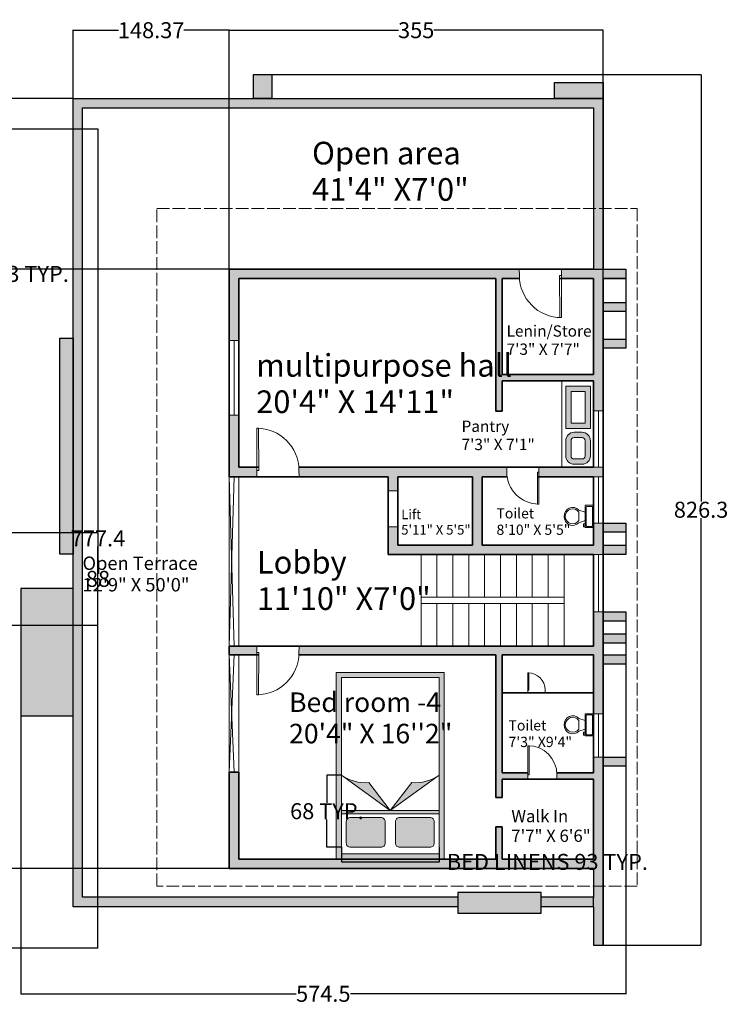
# Model space of a CAD drawing. Units: inches. Extents: x -828 to 1568, y -491 to 539.
# Tile 6 of 6: x 895 to 1568, y -470 to 464. Entities that reach past the tile are written whole.
import ezdxf

# ---------------------------------------------------------------- set-up
doc = ezdxf.new("R2010")
doc.units = ezdxf.units.IN
doc.header["$MEASUREMENT"] = 0
doc.linetypes.add('ACAD_ISO02W100', pattern=[15, 12, -3])
for name, color, linetype, lineweight in [('A-ANNO-DIMS', 2, 'Continuous', 18), ('A-AREA-IDEN', 7, 'Continuous', 18), ('A-DOOR', 3, 'Continuous', 18), ('A-FLOR-CASE', 9, 'Continuous', 18), ('A-FLOR-EVTR', 4, 'Continuous', 18), ('A-FLOR-FIXT', 9, 'Continuous', 18), ('A-FLOR-FIXT-PATT', 253, 'Continuous', 13), ('A-FLOR-SHFT', 7, 'Continuous', 25), ('A-FLOR-STRS', 7, 'Continuous', 18), ('A-FURN', 8, 'Continuous', 18), ('A-FURN-PATT', 253, 'Continuous', 13), ('A-GLAZ', 4, 'Continuous', 18), ('A-ROOF-OVHD', 8, 'ACAD_ISO02W100', 13), ('A-ROOF-PATT', 8, 'Continuous', 13), ('A-ROOF-PRPT', 7, 'Continuous', 25), ('A-WALL', 7, 'Continuous', 35), ('A-WALL-PATT', 8, 'Continuous', 13)]:
    doc.layers.add(name, color=color, linetype=linetype, lineweight=lineweight)
doc.styles.get("Standard").update_dxf_attribs({"font": 'arial.ttf'})
doc.dimstyles.get("Standard").update_dxf_attribs({"dimtxt": 15.18, "dimasz": 0.18, "dimexe": 0.18, "dimexo": 0.0625, "dimgap": 0.09, "dimtad": 0, "dimtih": 1, "dimtoh": 1, "dimdec": 0, "dimzin": 0, "dimdsep": 46, "dimlunit": 3, "dimtxsty": 'Standard', "dimcen": 0.09, "dimadec": 0, "dimazin": 0, "dimtfac": 1, "dimtdec": 0, "dimtofl": 0, "dimtmove": 0, "dimatfit": 3, "dimfxl": 1, "dimtolj": 1, "dimtzin": 0, "dimarcsym": 0})

# ---------------------------------------------------------------- blocks, each defined once
blk = doc.blocks.new('*U2')
for p, q in [((0, 0), (0, -6)), ((40, 0), (40, -6))]:
    blk.add_line(p, q)
blk.add_lwpolyline([(0, 0), (0, 40), (1.75, 40), (1.75, 0)], close=True)
blk.add_arc((0, 0), 40, 0, 90)
blk = doc.blocks.new('*U6')
for p, q in [((-10, -8.5), (-8, -8.5)), ((-10, -9.5), (-10, -8.5)), ((-8, -8.5), (-8, -8)), ((-7, -8), (-7, -9.5)), ((-4, -8), (-6, -14)), ((4, -8), (6, -14)), ((9.5, -6), (9.5, -2)), ((-7, -9.5), (-10, -9.5)), ((4, -14), (-4, -14))]:
    blk.add_line(p, q)
blk.add_lwpolyline([(10.5, -8), (10.5, 0), (-10.5, 0), (-10.5, -8)], close=True)
for points in [[(-9.5, -2), (-9.5, -6)], [(8.5, -1), (-8.5, -1)], [(-8.5, -7), (8.5, -7)]]:
    blk.add_lwpolyline(points)
for centre, radius, start, end in [((-8.625, -1.875), 0.8839, 81.8699, 188.1301), ((-8.625, -6.125), 0.8839, 171.869898, 278.1301), ((8.625, -1.875), 0.8839, 351.8699, 98.1301), ((8.625, -6.125), 0.8839, 261.8699, 8.1301), ((-0.4772, -19.9188), 8.0953, 133.01722, 273.38), ((0.0374, -19.8731), 7.127, 124.50543, 269.7), ((-0.0373, -19.8731), 7.127, 270.3, 55.4946), ((0.4773, -19.9188), 8.0953, 266.62, 46.9828)]:
    blk.add_arc(centre, radius, start, end)
blk = doc.blocks.new('BED-LINENS-DOUBLE')
h = blk.add_hatch(color=256)
h.dxf.hatch_style = 1
h.paths.add_polyline_path([(0, 92.62, -0.182673), (7.08, 66.8), (33.7, 46.31)])
h.paths.add_polyline_path([(33.7, 46.31), (7.08, 25.82, -0.182673), (0, 0)])
h = blk.add_hatch(color=256)
h.dxf.hatch_style = 1
h.paths.add_polyline_path([(36.7, 46.31), (33.7, 46.31), (33.7, 0), (36.7, 0)])
h.paths.add_polyline_path([(36.7, 92.62), (33.7, 92.62), (33.7, 46.31), (36.7, 46.31)])
h = blk.add_hatch(color=256)
h.dxf.hatch_style = 1
h.paths.add_polyline_path([(68.49, 84.07, 0.414214), (64.49, 88.07), (44.24, 88.07, 0.414214), (40.24, 84.07), (40.24, 55.21, 0.414214), (44.24, 51.21), (64.49, 51.21, 0.414214), (68.49, 55.21)])
h = blk.add_hatch(color=256)
h.dxf.hatch_style = 1
h.paths.add_polyline_path([(68.49, 37.42, 0.414214), (64.49, 41.42), (44.24, 41.42, 0.414214), (40.24, 37.42), (40.24, 8.55, 0.414214), (44.24, 4.55), (64.49, 4.55, 0.414214), (68.49, 8.55)])
for p, q in [((33.7, 46.31), (0, 92.62)), ((33.7, 0), (33.7, 92.62)), ((36.7, 0), (36.7, 92.62)), ((33.7, 46.31), (7.08, 66.8)), ((33.7, 46.31), (0, 0)), ((33.7, 46.31), (7.08, 25.82))]:
    blk.add_line(p, q)
for points in [[(64.49, 51.21), (44.24, 51.21, -0.414214), (40.24, 55.21), (40.24, 84.07, -0.414214), (44.24, 88.07), (64.49, 88.07, -0.414214), (68.49, 84.07), (68.49, 55.21, -0.414214)], [(64.49, 41.42), (44.24, 41.42, 0.414214), (40.24, 37.42), (40.24, 8.55, 0.414214), (44.24, 4.55), (64.49, 4.55, 0.414214), (68.49, 8.55), (68.49, 37.42, 0.414214)]]:
    blk.add_lwpolyline(points, format="xyb", close=True)
for centre, start, end in [((-30.62, 70.34), 354.63295, 36.04187), ((-30.62, 22.28), 323.95813, 5.36705)]:
    blk.add_arc(centre, 37.87, start, end)
blk = doc.blocks.new('*D25')
at = {"layer": 'A-ANNO-DIMS', "color": 0, "lineweight": -2, "transparency": 16777216}
for p, q in [((822.84, 244.58), (829.43, 244.58)), ((829.25, 244.4), (829.25, 230.97)), ((829.25, 201.64), (829.25, 215.08)), ((822.84, 201.46), (829.43, 201.46))]:
    blk.add_line(p, q, dxfattribs=at)
at = {"layer": 'A-ANNO-DIMS', "color": 0, "lineweight": 20, "transparency": 16777216}
for points in [[(829.22, 244.4), (829.28, 244.4), (829.25, 244.58)], [(829.22, 201.64), (829.28, 201.64), (829.25, 201.46)]]:
    blk.add_solid(points, dxfattribs=at)
at = {"layer": 'DEFPOINTS', "color": 0, "lineweight": 20, "transparency": 16777216}
for p in [(822.78, 244.58), (829.25, 244.58), (822.78, 201.46)]:
    blk.add_point(p, dxfattribs=at)
at = {"layer": 'A-ANNO-DIMS', "color": 0, "transparency": 16777216, "insert": (829.25, 223.02), "char_height": 15.18, "attachment_point": 5}
blk.add_mtext('\\A1;SERVICE SHAFT 43 TYP.', dxfattribs=at)
blk = doc.blocks.new('*D27')
at = {"layer": 'A-ANNO-DIMS', "color": 0, "lineweight": -2, "transparency": 16777216}
for p, q in [((1200.23, -321.25), (1200.23, -335.26)), ((1292.85, -321.25), (1292.85, -335.26)), ((1200.41, -335.08), (1292.67, -335.08)), ((1292.85, -335.08), (1293.03, -335.08))]:
    blk.add_line(p, q, dxfattribs=at)
at = {"layer": 'A-ANNO-DIMS', "color": 0, "lineweight": 20, "transparency": 16777216}
for points in [[(1200.41, -335.05), (1200.41, -335.11), (1200.23, -335.08)], [(1292.67, -335.05), (1292.67, -335.11), (1292.85, -335.08)]]:
    blk.add_solid(points, dxfattribs=at)
at = {"layer": 'DEFPOINTS', "color": 0, "lineweight": 20, "transparency": 16777216}
for p in [(1200.23, -321.18), (1292.85, -321.18), (1292.85, -335.08)]:
    blk.add_point(p, dxfattribs=at)
at = {"layer": 'A-ANNO-DIMS', "color": 0, "transparency": 16777216, "insert": (1395.73, -335.08), "char_height": 15.18, "attachment_point": 5}
blk.add_mtext('\\A1;BED LINENS 93 TYP.', dxfattribs=at)
blk = doc.blocks.new('*D28')
at = {"layer": 'A-ANNO-DIMS', "color": 0, "lineweight": -2, "transparency": 16777216}
for p, q in [((1200.17, -252.69), (1186.16, -252.69)), ((1186.34, -252.87), (1186.34, -279.1)), ((1186.34, -321), (1186.34, -294.78)), ((1200.17, -321.18), (1186.16, -321.18))]:
    blk.add_line(p, q, dxfattribs=at)
at = {"layer": 'A-ANNO-DIMS', "color": 0, "lineweight": 20, "transparency": 16777216}
for points in [[(1186.31, -252.87), (1186.37, -252.87), (1186.34, -252.69)], [(1186.31, -321), (1186.37, -321), (1186.34, -321.18)]]:
    blk.add_solid(points, dxfattribs=at)
at = {"layer": 'DEFPOINTS', "color": 0, "lineweight": 20, "transparency": 16777216}
for p in [(1200.23, -252.69), (1186.34, -321.18), (1200.23, -321.18)]:
    blk.add_point(p, dxfattribs=at)
at = {"layer": 'A-ANNO-DIMS', "color": 0, "transparency": 16777216, "insert": (1186.34, -286.94), "char_height": 15.18, "attachment_point": 5}
blk.add_mtext('\\A1;68 TYP.', dxfattribs=at)
blk = doc.blocks.new('*D40')
at = {"layer": 'A-ANNO-DIMS', "color": 0, "lineweight": -2, "transparency": 16777216}
for p, q in [((795.99, 360.63), (969.15, 360.63)), ((968.97, 360.45), (968.97, -20.38)), ((968.97, -416.57), (968.97, -35.74)), ((568.26, -416.75), (969.15, -416.75))]:
    blk.add_line(p, q, dxfattribs=at)
at = {"layer": 'A-ANNO-DIMS', "color": 0, "lineweight": 20, "transparency": 16777216}
for points in [[(968.94, 360.45), (969, 360.45), (968.97, 360.63)], [(968.94, -416.57), (969, -416.57), (968.97, -416.75)]]:
    blk.add_solid(points, dxfattribs=at)
at = {"layer": 'DEFPOINTS', "color": 0, "lineweight": 20, "transparency": 16777216}
for p in [(795.92, 360.63), (968.97, 360.63), (568.2, -416.75)]:
    blk.add_point(p, dxfattribs=at)
at = {"layer": 'A-ANNO-DIMS', "color": 0, "transparency": 16777216, "insert": (968.97, -28.06), "char_height": 15.18, "attachment_point": 5}
blk.add_mtext('\\A1;777.4', dxfattribs=at)
blk = doc.blocks.new('*D47')
at = {"layer": 'A-ANNO-DIMS', "color": 0, "lineweight": -2, "transparency": 16777216}
for p, q in [((786.99, -22.42), (969.15, -22.42)), ((968.97, -22.6), (968.97, -58.57)), ((968.97, -110.24), (968.97, -74.26)), ((786.99, -110.42), (969.15, -110.42))]:
    blk.add_line(p, q, dxfattribs=at)
at = {"layer": 'A-ANNO-DIMS', "color": 0, "lineweight": 20, "transparency": 16777216}
for points in [[(968.94, -22.6), (969, -22.6), (968.97, -22.42)], [(968.94, -110.24), (969, -110.24), (968.97, -110.42)]]:
    blk.add_solid(points, dxfattribs=at)
at = {"layer": 'DEFPOINTS', "color": 0, "lineweight": 20, "transparency": 16777216}
for p in [(786.92, -22.42), (968.97, -22.42), (786.92, -110.42)]:
    blk.add_point(p, dxfattribs=at)
at = {"layer": 'A-ANNO-DIMS', "color": 0, "transparency": 16777216, "insert": (968.97, -66.42), "char_height": 15.18, "attachment_point": 5}
blk.add_mtext('\\A1;88', dxfattribs=at)
blk = doc.blocks.new('*D49')
at = {"layer": 'A-ANNO-DIMS', "color": 0, "lineweight": -2, "transparency": 16777216}
for p, q in [((1470.21, -147.35), (1470.21, -460.48)), ((895.67, -196.43), (895.67, -460.48)), ((895.85, -460.3), (1157.18, -460.3)), ((1470.03, -460.3), (1208.7, -460.3))]:
    blk.add_line(p, q, dxfattribs=at)
at = {"layer": 'A-ANNO-DIMS', "color": 0, "lineweight": 20, "transparency": 16777216}
for points in [[(895.85, -460.27), (895.85, -460.33), (895.67, -460.3)], [(1470.03, -460.27), (1470.03, -460.33), (1470.21, -460.3)]]:
    blk.add_solid(points, dxfattribs=at)
at = {"layer": 'DEFPOINTS', "color": 0, "lineweight": 20, "transparency": 16777216}
for p in [(1470.21, -147.28), (895.67, -196.37), (1470.21, -460.3)]:
    blk.add_point(p, dxfattribs=at)
at = {"layer": 'A-ANNO-DIMS', "color": 0, "transparency": 16777216, "insert": (1182.94, -460.3), "char_height": 15.18, "attachment_point": 5}
blk.add_mtext('\\A1;574.5', dxfattribs=at)
blk = doc.blocks.new('*D50')
at = {"layer": 'A-ANNO-DIMS', "color": 0, "lineweight": -2, "transparency": 16777216}
for p, q in [((1116.69, 412.33), (1541.89, 412.33)), ((1541.71, 412.15), (1541.71, 7.03)), ((1541.71, -413.79), (1541.71, -8.66)), ((1448.72, -413.97), (1541.89, -413.97))]:
    blk.add_line(p, q, dxfattribs=at)
at = {"layer": 'A-ANNO-DIMS', "color": 0, "lineweight": 20, "transparency": 16777216}
for points in [[(1541.68, 412.15), (1541.74, 412.15), (1541.71, 412.33)], [(1541.68, -413.79), (1541.74, -413.79), (1541.71, -413.97)]]:
    blk.add_solid(points, dxfattribs=at)
at = {"layer": 'DEFPOINTS', "color": 0, "lineweight": 20, "transparency": 16777216}
for p in [(1116.62, 412.33), (1541.71, 412.33), (1448.66, -413.97)]:
    blk.add_point(p, dxfattribs=at)
at = {"layer": 'A-ANNO-DIMS', "color": 0, "transparency": 16777216, "insert": (1541.71, -0.82), "char_height": 15.18, "attachment_point": 5}
blk.add_mtext('\\A1;826.3', dxfattribs=at)
blk = doc.blocks.new('*D51')
at = {"layer": 'A-ANNO-DIMS', "color": 0, "lineweight": -2, "transparency": 16777216}
for p, q in [((945.29, 389.64), (945.29, 454.56)), ((945.47, 454.38), (988.59, 454.38)), ((1093.48, 454.38), (1050.36, 454.38)), ((1093.66, 227.62), (1093.66, 454.56))]:
    blk.add_line(p, q, dxfattribs=at)
at = {"layer": 'A-ANNO-DIMS', "color": 0, "lineweight": 20, "transparency": 16777216}
for points in [[(945.47, 454.41), (945.47, 454.35), (945.29, 454.38)], [(1093.48, 454.41), (1093.48, 454.35), (1093.66, 454.38)]]:
    blk.add_solid(points, dxfattribs=at)
at = {"layer": 'DEFPOINTS', "color": 0, "lineweight": 20, "transparency": 16777216}
for p in [(1093.66, 454.38), (945.29, 389.57), (1093.66, 227.56)]:
    blk.add_point(p, dxfattribs=at)
at = {"layer": 'A-ANNO-DIMS', "color": 0, "transparency": 16777216, "insert": (1019.47, 454.38), "char_height": 15.18, "attachment_point": 5}
blk.add_mtext('\\A1;148.37', dxfattribs=at)
blk = doc.blocks.new('*D52')
at = {"layer": 'A-ANNO-DIMS', "color": 0, "lineweight": -2, "transparency": 16777216}
for p, q in [((1093.66, 227.62), (1093.66, 454.56)), ((1093.84, 454.38), (1254.25, 454.38)), ((1448.48, 454.38), (1288.07, 454.38)), ((1448.66, 227.62), (1448.66, 454.56))]:
    blk.add_line(p, q, dxfattribs=at)
at = {"layer": 'A-ANNO-DIMS', "color": 0, "lineweight": 20, "transparency": 16777216}
for points in [[(1093.84, 454.41), (1093.84, 454.35), (1093.66, 454.38)], [(1448.48, 454.41), (1448.48, 454.35), (1448.66, 454.38)]]:
    blk.add_solid(points, dxfattribs=at)
at = {"layer": 'DEFPOINTS', "color": 0, "lineweight": 20, "transparency": 16777216}
for p in [(1448.66, 454.38), (1093.66, 227.56), (1448.66, 227.56)]:
    blk.add_point(p, dxfattribs=at)
at = {"layer": 'A-ANNO-DIMS', "color": 0, "transparency": 16777216, "insert": (1271.16, 454.38), "char_height": 15.18, "attachment_point": 5}
blk.add_mtext('\\A1;355', dxfattribs=at)
blk = doc.blocks.new('*D53')
at = {"layer": 'A-ANNO-DIMS', "color": 0, "lineweight": -2, "transparency": 16777216}
for p, q in [((945.23, 389.57), (846.26, 389.57)), ((846.44, 389.39), (846.44, 316.41)), ((846.44, 227.74), (846.44, 300.73)), ((1093.6, 227.56), (846.26, 227.56))]:
    blk.add_line(p, q, dxfattribs=at)
at = {"layer": 'A-ANNO-DIMS', "color": 0, "lineweight": 20, "transparency": 16777216}
for points in [[(846.41, 389.39), (846.47, 389.39), (846.44, 389.57)], [(846.41, 227.74), (846.47, 227.74), (846.44, 227.56)]]:
    blk.add_solid(points, dxfattribs=at)
at = {"layer": 'DEFPOINTS', "color": 0, "lineweight": 20, "transparency": 16777216}
for p in [(945.29, 389.57), (846.44, 227.56), (1093.66, 227.56)]:
    blk.add_point(p, dxfattribs=at)
at = {"layer": 'A-ANNO-DIMS', "color": 0, "transparency": 16777216, "insert": (846.44, 308.57), "char_height": 15.18, "attachment_point": 5}
blk.add_mtext('\\A1;162', dxfattribs=at)
blk = doc.blocks.new('*D54')
at = {"layer": 'A-ANNO-DIMS', "color": 0, "lineweight": -2, "transparency": 16777216}
for p, q in [((1093.6, 227.56), (846.26, 227.56)), ((846.44, 227.38), (846.44, -49.1)), ((846.44, -341.26), (846.44, -64.78)), ((1093.6, -341.44), (846.26, -341.44))]:
    blk.add_line(p, q, dxfattribs=at)
at = {"layer": 'A-ANNO-DIMS', "color": 0, "lineweight": 20, "transparency": 16777216}
for points in [[(846.41, 227.38), (846.47, 227.38), (846.44, 227.56)], [(846.41, -341.26), (846.47, -341.26), (846.44, -341.44)]]:
    blk.add_solid(points, dxfattribs=at)
at = {"layer": 'DEFPOINTS', "color": 0, "lineweight": 20, "transparency": 16777216}
for p in [(846.44, 227.56), (1093.66, 227.56), (1093.66, -341.44)]:
    blk.add_point(p, dxfattribs=at)
at = {"layer": 'A-ANNO-DIMS', "color": 0, "transparency": 16777216, "insert": (846.44, -56.94), "char_height": 15.18, "attachment_point": 5}
blk.add_mtext('\\A1;569', dxfattribs=at)

msp = doc.modelspace()

# ---------------------------------------------------------------- hatches: boundary and pattern name
at = {"layer": 'A-FLOR-FIXT-PATT'}
h = msp.add_hatch(color=256, dxfattribs=at)
h.dxf.hatch_style = 1
h.paths.add_polyline_path([(1436.6542, 76.4323), (1436.6542, 116.4537), (1413.21, 116.4537), (1413.21, 76.4323)])
h.paths.add_polyline_path([(1431.6542, 81.4323), (1418.21, 81.4323), (1418.21, 111.4537), (1431.6542, 111.4537)], flags=16)
h.paths.add_polyline_path([(1436.6542, 64.7082, 0.41421356), (1428.6542, 72.7082), (1421.21, 72.7082, 0.41421356), (1413.21, 64.7082), (1413.21, 50.408, 0.41421356), (1421.21, 42.408), (1428.6542, 42.408, 0.41421356), (1436.6542, 50.408)])
h.paths.add_polyline_path([(1431.6542, 50.408, -0.41421356), (1428.6542, 47.408), (1421.21, 47.408, -0.41421356), (1418.21, 50.408), (1418.21, 64.7082, -0.41421356), (1421.21, 67.7082), (1428.6542, 67.7082, -0.41421356), (1431.6542, 64.7082)], flags=16)
at = {"layer": 'A-FURN-PATT'}
h = msp.add_hatch(color=256, dxfattribs=at)
h.dxf.hatch_style = 1
h.paths.add_polyline_path([(1195.2304, -155.182), (1195.2304, -332.4397), (1297.8521, -332.4397), (1297.8521, -155.182)])
h.paths.add_polyline_path([(1292.8521, -160.182), (1292.8521, -327.4397), (1200.2304, -327.4397), (1200.2304, -160.182)], flags=16)
at = {"layer": 'A-ROOF-PATT'}
h = msp.add_hatch(color=256, dxfattribs=at)
h.dxf.hatch_style = 1
h.paths.add_polyline_path([(1448.6584, 404.7457), (1402.3549, 404.7457), (1402.3549, 389.5728), (1448.6584, 389.5728)])
h.paths.add_polyline_path([(1134.1815, 412.3327), (1116.6243, 412.3327), (1116.6243, 389.5728), (1134.1815, 389.5728)])
h.paths.add_polyline_path([(1448.6584, 284.9999), (1439.6584, 284.9999), (1439.6584, 227.5603), (1448.6584, 227.5603)], flags=17)
h.paths.add_polyline_path([(945.2883, -75.6073), (895.6713, -75.6073), (895.6713, -196.3658), (945.2883, -196.3658)])
h.paths.add_polyline_path([(945.2883, 161.9328), (932.8692, 161.9328), (932.8692, -42.8816), (945.2883, -42.8816)])
h.paths.add_polyline_path([(954.2883, 380.5728), (1439.6584, 380.5728), (1439.6584, 284.9999), (1448.6584, 284.9999), (1448.6584, 389.5728), (1402.3549, 389.5728), (945.2883, 389.5728), (945.2883, -377.7023), (1310.7371, -377.7023), (1310.7371, -368.7023), (954.2883, -368.7023)])
h = msp.add_hatch(color=256, dxfattribs=at)
h.dxf.hatch_style = 1
h.paths.add_polyline_path([(1389.6889, -364.1494), (1310.7371, -364.1494), (1310.7371, -383.7147), (1389.6889, -383.7147)])
h.paths.add_polyline_path([(1439.6584, -368.7023), (1389.6889, -368.7023), (1389.6889, -377.7023), (1439.6584, -377.7023)])
at = {"layer": 'A-WALL-PATT'}
h = msp.add_hatch(color=256, dxfattribs=at)
h.dxf.hatch_style = 1
h.paths.add_polyline_path([(1448.6584, 227.5603), (1439.6584, 227.5603), (1409.1076, 227.5603), (1409.1183, 221.5603), (1409.1236, 218.5603), (1439.6584, 218.5603), (1439.6584, 127.5603), (1352.6584, 127.5603), (1352.6584, 218.5603), (1369.2309, 218.5603, -0.01832557), (1369.1183, 221.4893), (1369.1075, 227.5603), (1093.6584, 227.5603), (1093.6584, 159.8045), (1102.6584, 159.8045), (1102.6584, 218.5603), (1346.6584, 218.5603), (1346.6584, 127.5603), (1346.6584, 92.5995), (1352.6584, 92.5995), (1352.6584, 121.5603), (1439.6584, 121.5603), (1439.6584, 92.9827), (1448.6584, 92.9827), (1448.6584, 218.2927), (1470.211, 218.2927), (1470.211, 218.8223), (1448.6584, 218.8223)])
h.paths.add_polyline_path([(1470.211, 161.1899), (1448.6584, 161.1899), (1448.6584, 152.4519), (1470.211, 152.4519)], flags=17)
h.paths.add_polyline_path([(1470.211, 196.0219), (1448.6584, 196.0219), (1448.6584, 187.2839), (1470.211, 187.2839)], flags=17)
h.paths.add_polyline_path([(1470.211, 227.5603), (1448.6584, 227.5603), (1448.6584, 218.8223), (1470.211, 218.8223)], flags=17)
h.paths.add_polyline_path([(1448.6584, -357.9803), (1439.6584, -357.9803), (1439.6584, -368.7023), (1439.6584, -377.7023), (1439.6584, -413.965), (1448.6584, -413.965)])
h.paths.add_polyline_path([(1470.211, -235.5345), (1448.6584, -235.5345), (1448.6584, -244.2725), (1470.211, -244.2725)])
h.paths.add_polyline_path([(1470.211, -118.6948), (1448.6584, -118.6948), (1448.6584, -127.4328), (1470.211, -127.4328)])
h.paths.add_polyline_path([(1470.211, -138.5447), (1448.6584, -138.5447), (1448.6584, -147.2827), (1470.211, -147.2827)])
h.paths.add_polyline_path([(1470.211, -97.8361), (1448.6584, -97.8361), (1448.6584, -106.5741), (1470.211, -106.5741)])
h.paths.add_polyline_path([(1470.211, -13.468), (1448.6584, -13.468), (1448.6584, -22.2061), (1470.211, -22.2061)])
h.paths.add_polyline_path([(1470.211, -34.4241), (1448.6584, -34.4241), (1448.6584, -43.1621), (1470.211, -43.1621)])
h.paths.add_polyline_path([(1357.1129, 34.9933), (1357.1129, 39.5603), (1159.7541, 39.5603, -0.01832557), (1159.8667, 36.6314), (1159.8775, 30.5603), (1244.6584, 30.5603), (1244.6584, 17.0889), (1253.6584, 17.0889), (1253.6584, 30.5603), (1324.6584, 30.5603), (1324.6584, -34.4397), (1253.6584, -34.4397), (1253.6584, -16.894), (1244.6584, -16.894), (1244.6584, -43.4397), (1439.6584, -43.4397), (1448.6584, -43.4397), (1448.6584, -43.1621), (1448.6584, -34.4241), (1448.6584, -13.468), (1439.6584, -13.468), (1439.6584, -17.6159), (1439.6584, -34.4397), (1333.6584, -34.4397), (1333.6584, 30.5603), (1357.4374, 30.5603, -0.03654584)])
h.paths.add_polyline_path([(1448.6584, 39.5603), (1439.6584, 39.5603), (1409.6286, 39.5603), (1387.5596, 39.5603), (1387.5596, 34.9933), (1387.5596, 30.5603), (1439.6584, 30.5603), (1448.6584, 30.5603)], flags=17)
h.paths.add_polyline_path([(1119.8614, 39.5603), (1102.6584, 39.5603), (1102.6584, 88.8742), (1098.1584, 88.8742), (1093.6584, 88.8742), (1093.6584, 30.5603), (1098.1584, 30.5603), (1102.6584, 30.5603), (1119.8774, 30.5603), (1119.8668, 36.5603)])
h.paths.add_polyline_path([(1448.6584, -97.8361), (1439.6584, -97.8361), (1439.6584, -130.4397), (1159.8775, -130.4397), (1159.8667, -136.5107, -0.01206169), (1159.8167, -138.4397), (1346.6584, -138.4397), (1346.6584, -273.9049), (1352.6584, -273.9049), (1352.6584, -256.4397), (1377.2942, -256.4397), (1377.2868, -252.3087), (1377.2835, -250.4397), (1352.6584, -250.4397), (1352.6584, -138.4397), (1439.6584, -138.4397), (1439.6584, -194.4397), (1448.6584, -194.4397)])
h.paths.add_polyline_path([(1119.8774, -130.4397), (1093.6584, -130.4397), (1093.6584, -138.4397), (1098.1584, -138.4397), (1102.6584, -138.4397), (1119.8632, -138.4397), (1119.8668, -136.4397)])
h.paths.add_polyline_path([(1448.6584, -235.5345), (1439.6584, -235.5345), (1439.6584, -250.4397), (1404.7632, -250.4397, -0.01653697), (1404.8266, -252.2598), (1404.8341, -256.4397), (1439.6584, -256.4397), (1439.6584, -332.4397), (1352.6584, -332.4397), (1352.6584, -301.8354), (1346.6584, -301.8354), (1346.6584, -332.4397), (1102.6584, -332.4397), (1102.6584, -249.8688), (1093.6584, -249.8688), (1093.6584, -341.4397), (1439.6584, -341.4397), (1439.6584, -357.9803), (1448.6584, -357.9803)])

# ---------------------------------------------------------------- linework, layer by layer
at = {"layer": 'A-FLOR-CASE'}
msp.add_lwpolyline([(1439.6584, 39.5603), (1409.6286, 39.5603), (1409.6286, 121.5603), (1439.6584, 121.5603)], close=True, dxfattribs=at)
at = {"layer": 'A-FLOR-EVTR'}
msp.add_lwpolyline([(1253.6584, -16.894), (1244.6584, -16.894), (1244.6584, 17.0889), (1253.6584, 17.0889)], close=True, dxfattribs=at)
at = {"layer": 'A-FLOR-FIXT'}
for points in [[(1413.21, 116.4537), (1436.6542, 116.4537), (1436.6542, 76.4323), (1413.21, 76.4323)], [(1418.21, 111.4537), (1431.6542, 111.4537), (1431.6542, 81.4323), (1418.21, 81.4323)]]:
    msp.add_lwpolyline(points, close=True, dxfattribs=at)
for points in [[(1421.21, 72.7082), (1428.6542, 72.7082, -0.41421356), (1436.6542, 64.7082), (1436.6542, 50.408, -0.41421356), (1428.6542, 42.408), (1421.21, 42.408, -0.41421356), (1413.21, 50.408), (1413.21, 64.7082, -0.41421356)], [(1421.21, 67.7082), (1428.6542, 67.7082, -0.41421356), (1431.6542, 64.7082), (1431.6542, 50.408, -0.41421356), (1428.6542, 47.408), (1421.21, 47.408, -0.41421356), (1418.21, 50.408), (1418.21, 64.7082, -0.41421356)]]:
    msp.add_lwpolyline(points, format="xyb", close=True, dxfattribs=at)
at = {"layer": 'A-FLOR-SHFT'}
for p, q in [((1439.6584, 227.5603), (1470.211, 227.5603)), ((1470.211, 227.5603), (1470.211, 218.2927)), ((1470.211, 227.5603), (1470.211, 152.4519)), ((1470.211, 218.2927), (1448.6584, 218.2927)), ((1470.211, -13.468), (1470.211, -43.1621)), ((1470.211, -97.8361), (1470.211, -147.2827))]:
    msp.add_line(p, q, dxfattribs=at)
for points in [[(1448.6584, 227.5603), (1470.211, 227.5603), (1470.211, 218.8223), (1448.6584, 218.8223)], [(1448.6584, 196.0219), (1470.211, 196.0219), (1470.211, 187.2839), (1448.6584, 187.2839)], [(1448.6584, 161.1899), (1470.211, 161.1899), (1470.211, 152.4519), (1448.6584, 152.4519)], [(1448.6584, -13.468), (1470.211, -13.468), (1470.211, -22.2061), (1448.6584, -22.2061)], [(1448.6584, -34.4241), (1470.211, -34.4241), (1470.211, -43.1621), (1448.6584, -43.1621)], [(1448.6584, -97.8361), (1470.211, -97.8361), (1470.211, -106.5741), (1448.6584, -106.5741)], [(1448.6584, -118.6948), (1470.211, -118.6948), (1470.211, -127.4328), (1448.6584, -127.4328)], [(1448.6584, -138.5447), (1470.211, -138.5447), (1470.211, -147.2827), (1448.6584, -147.2827)], [(1448.6584, -235.5345), (1470.211, -235.5345), (1470.211, -244.2725), (1448.6584, -244.2725)]]:
    msp.add_lwpolyline(points, close=True, dxfattribs=at)
at = {"layer": 'A-FLOR-STRS'}
for p, q in [((1275.7589, -43.4397), (1275.7589, -130.4397)), ((1290.8578, -43.4397), (1290.8578, -83.9397)), ((1305.9568, -43.4397), (1305.9568, -83.9397)), ((1321.0557, -43.4397), (1321.0557, -83.9397)), ((1336.1546, -43.4397), (1336.1546, -83.9397)), ((1351.2535, -43.4397), (1351.2535, -83.9397)), ((1366.3524, -43.4397), (1366.3524, -83.9397)), ((1381.4513, -43.4397), (1381.4513, -83.9397)), ((1396.5502, -43.4397), (1396.5502, -83.9397)), ((1411.6491, -86.9397), (1411.6491, -43.4397)), ((1411.6491, -43.4397), (1411.6491, -130.4397)), ((1411.6491, -43.4397), (1411.6491, -130.4397)), ((1275.7589, -83.9397), (1411.6491, -83.9397)), ((1275.7589, -89.9397), (1411.6491, -89.9397)), ((1290.8578, -89.9397), (1290.8578, -130.4397)), ((1305.9568, -89.9397), (1305.9568, -130.4397)), ((1321.0557, -89.9397), (1321.0557, -130.4397)), ((1336.1546, -89.9397), (1336.1546, -130.4397)), ((1351.2535, -89.9397), (1351.2535, -130.4397)), ((1366.3524, -89.9397), (1366.3524, -130.4397)), ((1381.4513, -89.9397), (1381.4513, -130.4397)), ((1396.5502, -89.9397), (1396.5502, -130.4397))]:
    msp.add_line(p, q, dxfattribs=at)
at = {"layer": 'A-FURN'}
for points in [[(1195.2304, -332.4397), (1195.2304, -155.182), (1297.8521, -155.182), (1297.8521, -332.4397)], [(1200.2304, -327.4397), (1200.2304, -160.182), (1292.8521, -160.182), (1292.8521, -327.4397)]]:
    msp.add_lwpolyline(points, close=True, dxfattribs=at)
at = {"layer": 'A-GLAZ'}
for p, q in [((1093.6584, 88.8742), (1093.6584, 159.8045)), ((1093.6584, 159.8045), (1102.6584, 159.8045)), ((1098.1584, 88.8742), (1098.1584, 159.8045)), ((1102.6584, 159.8045), (1102.6584, 88.8742)), ((1102.6584, 88.8742), (1093.6584, 88.8742)), ((1102.6584, 88.8742), (1098.1584, 88.8742)), ((1444.1584, 92.9827), (1444.1584, 39.5603)), ((1098.1584, -130.4397), (1093.6584, 30.5603)), ((1093.6584, 30.5603), (1098.1584, 30.5603)), ((1098.1584, 30.5603), (1093.6584, -130.4397)), ((1444.1584, -13.468), (1444.1584, 30.5603)), ((1444.1584, -43.4397), (1444.1584, -97.8361)), ((1098.1584, -249.8688), (1093.6584, -138.4397)), ((1093.6584, -138.4397), (1098.1584, -138.4397)), ((1098.1584, -138.4397), (1093.6584, -249.8688)), ((1444.1584, -235.5345), (1444.1584, -194.4397))]:
    msp.add_line(p, q, dxfattribs=at)
for points in [[(1448.6584, 39.5603), (1439.6584, 39.5603), (1439.6584, 92.9827), (1448.6584, 92.9827)], [(1093.6584, -130.4397), (1102.6584, -130.4397), (1102.6584, 30.5603), (1093.6584, 30.5603)], [(1439.6584, 30.5603), (1448.6584, 30.5603), (1448.6584, -13.468), (1439.6584, -13.468)], [(1439.6584, -43.4397), (1448.6584, -43.4397), (1448.6584, -97.8361), (1439.6584, -97.8361)], [(1102.6584, -249.8688), (1093.6584, -249.8688), (1093.6584, -138.4397), (1102.6584, -138.4397)], [(1448.6584, -235.5345), (1439.6584, -235.5345), (1439.6584, -194.4397), (1448.6584, -194.4397)]]:
    msp.add_lwpolyline(points, close=True, dxfattribs=at)
at = {"layer": 'A-ROOF-OVHD'}
msp.add_lwpolyline([(1024.7823, 284.9999), (1480.9966, 284.9999), (1480.9966, -357.9803), (1024.7823, -357.9803)], close=True, dxfattribs=at)
at = {"layer": 'A-ROOF-PRPT'}
for p, q in [((945.2883, -377.7023), (945.2883, 389.5728)), ((945.2883, 389.5728), (1448.6584, 389.5728)), ((1448.6584, 389.5728), (1448.6584, 227.5603)), ((954.2883, -368.7023), (954.2883, 380.5728)), ((954.2883, 380.5728), (1439.6584, 380.5728)), ((1439.6584, 380.5728), (1439.6584, 227.5603)), ((1439.6584, -341.4397), (1439.6584, -368.7023)), ((1310.7371, -368.7023), (954.2883, -368.7023)), ((1439.6584, -368.7023), (1389.6889, -368.7023)), ((1439.6584, -377.7023), (1439.6584, -368.7023)), ((1310.7371, -377.7023), (945.2883, -377.7023)), ((1439.6584, -377.7023), (1389.6889, -377.7023)), ((1439.6584, -377.7023), (1439.6584, -413.965)), ((1439.6584, -413.965), (1448.6584, -413.965))]:
    msp.add_line(p, q, dxfattribs=at)
for points in [[(1134.1815, 389.5728), (1116.6243, 389.5728), (1116.6243, 412.3327), (1134.1815, 412.3327)], [(1448.6584, 389.5728), (1402.3549, 389.5728), (1402.3549, 404.7457), (1448.6584, 404.7457)], [(945.2883, -42.8816), (932.8692, -42.8816), (932.8692, 161.9328), (945.2883, 161.9328)], [(945.2883, -75.6073), (895.6713, -75.6073), (895.6713, -196.3658), (945.2883, -196.3658)], [(1389.6889, -364.1494), (1310.7371, -364.1494), (1310.7371, -383.7147), (1389.6889, -383.7147)]]:
    msp.add_lwpolyline(points, close=True, dxfattribs=at)
at = {"layer": 'A-WALL'}
for p, q in [((1439.6584, 227.5603), (1093.6584, 227.5603)), ((1093.6584, 227.5603), (1093.6584, 30.5603)), ((1346.6584, 218.5603), (1102.6584, 218.5603)), ((1346.6584, 218.5603), (1102.6584, 218.5603)), ((1102.6584, 218.5603), (1102.6584, 218.5603)), ((1102.6584, 218.5603), (1102.6584, 39.5603)), ((1346.6584, 127.5603), (1346.6584, 218.5603)), ((1352.6584, 127.5603), (1352.6584, 218.5603)), ((1369.2309, 218.5603), (1352.6584, 218.5603)), ((1439.6584, 218.5603), (1407.3736, 218.5603)), ((1439.6584, 218.5603), (1439.6584, 127.5603)), ((1439.6584, 127.5603), (1439.6584, 218.5603)), ((1448.6584, 218.2927), (1448.6584, -413.965)), ((1346.6584, 112.2613), (1346.6584, 127.5603)), ((1346.6584, 127.5603), (1346.6584, 92.5995)), ((1439.6584, 127.5603), (1352.6584, 127.5603)), ((1439.6584, 121.5603), (1352.6584, 121.5603)), ((1352.6584, 121.5603), (1352.6584, 92.5995)), ((1439.6584, 127.5603), (1439.6584, 127.5603)), ((1439.6584, 39.5603), (1439.6584, 121.5603)), ((1352.6584, 92.5995), (1346.6584, 92.5995)), ((1121.6114, 39.5603), (1102.6584, 39.5603)), ((1439.6584, 39.5603), (1159.7541, 39.5603)), ((1244.6584, 30.5603), (1093.6584, 30.5603)), ((1244.6584, 30.5603), (1244.6584, -43.4397)), ((1253.6584, 30.5603), (1253.6584, -34.4397)), ((1324.6584, 30.5603), (1253.6584, 30.5603)), ((1324.6584, 30.5603), (1324.6584, -34.4397)), ((1333.6584, 30.5603), (1333.6584, -34.4397)), ((1357.4374, 30.5603), (1333.6584, 30.5603)), ((1439.6584, 30.5603), (1386.2276, 30.5603)), ((1439.6584, 30.5603), (1439.6584, -34.4397)), ((1324.6584, -34.4397), (1253.6584, -34.4397)), ((1439.6584, -34.4397), (1333.6584, -34.4397)), ((1439.6584, -43.4397), (1244.6584, -43.4397)), ((1439.6584, -43.4397), (1439.6584, -130.4397)), ((1439.6584, -130.4397), (1093.6584, -130.4397)), ((1093.6584, -130.4397), (1093.6584, -138.4397)), ((1121.6132, -138.4397), (1093.6584, -138.4397)), ((1346.6584, -138.4397), (1159.8167, -138.4397)), ((1346.6584, -138.4397), (1346.6584, -273.9049)), ((1439.6584, -138.4397), (1352.6584, -138.4397)), ((1352.6584, -138.4397), (1352.6584, -250.4397)), ((1439.6584, -138.4397), (1439.6584, -250.4397)), ((1352.6584, -174.4498), (1439.6584, -174.4498)), ((1102.6584, -249.8688), (1093.6584, -249.8688)), ((1093.6584, -249.8688), (1093.6584, -341.4397)), ((1102.6584, -332.4397), (1102.6584, -249.8688)), ((1377.2888, -250.4397), (1352.6584, -250.4397)), ((1439.6584, -250.4397), (1404.7632, -250.4397)), ((1439.6584, -256.4397), (1352.6584, -256.4397)), ((1352.6584, -256.4397), (1352.6584, -273.9049)), ((1439.6584, -256.4397), (1439.6584, -332.4397)), ((1352.6584, -273.9049), (1346.6584, -273.9049)), ((1346.6584, -301.8354), (1352.6584, -301.8354)), ((1346.6584, -301.8354), (1346.6584, -332.4397)), ((1352.6584, -301.8354), (1352.6584, -332.4397)), ((1346.6584, -332.4397), (1102.6584, -332.4397)), ((1439.6584, -332.4397), (1352.6584, -332.4397)), ((1439.6584, -341.4397), (1093.6584, -341.4397))]:
    msp.add_line(p, q, dxfattribs=at)

# ---------------------------------------------------------------- block references
at = {"layer": 'A-DOOR'}
for p, rotation in [((1409.1183, 221.5603), 180.1017956641893), ((1119.8668, 36.5603), 0.1017956641893213)]:
    msp.add_blockref('*U2', p, dxfattribs=dict(at, rotation=rotation))
for p, xscale, yscale, zscale, rotation in [((1387.5596, 34.9933), 0.7611664892927207, 0.7611664892927207, 0.7611664892927207, 180), ((1377.2898, -171.9823), 0.4112466119041872, 0.4112466119041872, 0.4112466119041872, 0.1017956641893213), ((1377.2868, -252.3087), 0.6884963100634148, 0.6884963100634148, 0.6884963100634148, 0.1017956641893213)]:
    msp.add_blockref('*U2', p, dxfattribs=dict(at, xscale=xscale, yscale=yscale, zscale=zscale, rotation=rotation))
at = {"layer": 'A-DOOR', "xscale": -1, "rotation": 179.8982043358106}
msp.add_blockref('*U2', (1119.8668, -136.4397), dxfattribs=at)
at = {"layer": 'A-FLOR-FIXT', "xscale": -1, "rotation": 270}
for p in [(1439.6584, -7.1159), (1439.6584, -204.9397)]:
    msp.add_blockref('*U6', p, dxfattribs=at)
at = {"layer": 'A-FURN', "rotation": 270}
msp.add_blockref('BED-LINENS-DOUBLE', (1200.2306, -252.6888), dxfattribs=at)

# ---------------------------------------------------------------- texts
at = {"layer": 'A-AREA-IDEN'}
for s, height, p in [('Open area', 21.48987, (1172.2547, 326.9638)), ('41\'4" X7\'0"', 21.489868, (1172.2547, 292.4422)), ('Lenin/Store', 10.746372, (1356.9895, 163.4738)), ('7\'3" X 7\'7"', 10.746372, (1356.9895, 146.2107)), ('multipurpose hall', 21.489868, (1119.1851, 125.4744)), ('20\'4" X 14\'11"', 21.489868, (1119.1851, 90.9528)), ('Pantry', 10.74637, (1314.2116, 73.0544)), ('7\'3" X 7\'1"', 10.746372, (1314.2116, 55.7913)), ('Lift', 9.11352, (1256.9303, -9.7671)), ('Toilet', 9.69979, (1347.452, -9.0536)), ('5\'11" X 5\'5"', 9.113515, (1256.9303, -24.4071)), ('8\'10" X 5\'5"', 9.699787, (1347.452, -24.6355)), ('Open Terrace', 12.720619, (954.2883, -57.9258)), ('Lobby', 21.48987, (1119.8774, -61.3965)), ('12\'9" X 50\'0"', 12.720619, (954.2883, -78.3603)), ('11\'10" X7\'0"', 21.489868, (1119.8774, -95.9181)), ('Bed room -4', 18.535465, (1150.4194, -192.7669)), ('20\'4" X 16\'\'2"', 18.535465, (1150.4194, -222.5424)), ('Toilet', 9.78566, (1358.8113, -210.3589)), ('7\'3" X9\'4"', 9.78566, (1358.8113, -226.0787)), ('Walk In', 11.63279, (1361.5162, -297.426)), ('7\'7" X 6\'6"', 11.632794, (1361.5162, -316.1131))]:
    msp.add_text(s, height=height, dxfattribs=at).set_placement(p)

# ---------------------------------------------------------------- dimensions: what is measured, and where the dimension line sits
at = {"layer": 'A-ANNO-DIMS'}
for base, p1, p2, override, picture, middle in [((1093.6584, 454.3827), (945.2883, 389.5728), (1093.6584, 227.5603), {"dimdec": 2, "dimlfac": 1, "dimrnd": 0, "dimzin": 0, "dimdsep": 46, "dimlunit": 2}, '*D51', (1019.4733, 454.3827)), ((1448.6584, 454.3827), (1093.6584, 227.5603), (1448.6584, 227.5603), {"dimdec": 0, "dimlfac": 1, "dimrnd": 0, "dimzin": 0, "dimdsep": 46, "dimlunit": 2}, '*D52', (1271.1584, 454.3827)), ((1470.211, -460.2973), (895.6713, -196.3658), (1470.211, -147.2827), {"dimdec": 1, "dimlfac": 1, "dimrnd": 0, "dimzin": 0, "dimdsep": 46, "dimlunit": 2}, '*D49', (1182.9411, -460.2973))]:
    dim = msp.add_linear_dim(base=base, p1=p1, p2=p2, dimstyle='Standard', override=override, dxfattribs=at)
    dim.commit()
    dim.dimension.update_dxf_attribs({"geometry": picture, "text_midpoint": middle})
for base, p1, p2, override, picture, middle in [((1541.7084, 412.3327), (1448.6584, -413.965), (1116.6243, 412.3327), {"dimdec": 1, "dimlfac": 1, "dimrnd": 0, "dimzin": 0, "dimdsep": 46, "dimlunit": 2}, '*D50', (1541.7084, -0.8162)), ((846.4381, 227.5603), (945.2883, 389.5728), (1093.6584, 227.5603), {"dimdec": 0, "dimlfac": 1, "dimrnd": 0, "dimzin": 0, "dimdsep": 46, "dimlunit": 2}, '*D53', (846.4381, 308.5666)), ((968.971, 360.6319), (568.196, -416.7473), (795.9226, 360.6319), {"dimdec": 1, "dimlfac": 1, "dimrnd": 0, "dimzin": 0, "dimdsep": 46, "dimlunit": 2}, '*D40', (968.971, -28.0577)), ((846.4381, 227.5603), (1093.6584, -341.4397), (1093.6584, 227.5603), {"dimdec": 0, "dimlfac": 1, "dimrnd": 0, "dimzin": 0, "dimdsep": 46, "dimlunit": 2}, '*D54', (846.4381, -56.9397)), ((968.971, -22.4155), (786.9226, -110.4155), (786.9226, -22.4155), {"dimdec": 0, "dimlfac": 1, "dimrnd": 0, "dimzin": 0, "dimdsep": 46, "dimlunit": 2}, '*D47', (968.971, -66.4155))]:
    dim = msp.add_linear_dim(base=base, p1=p1, p2=p2, angle=90, dimstyle='Standard', override=override, dxfattribs=at)
    dim.commit()
    dim.dimension.update_dxf_attribs({"geometry": picture, "text_midpoint": middle})
for base, p1, p2, angle, text, picture, middle in [((829.2484, 244.5845), (822.7802, 201.4634), (822.7802, 244.5845), 90, 'SERVICE SHAFT <> TYP.', '*D25', (829.2484, 223.0239)), ((1186.3372, -321.1831), (1200.2304, -252.6889), (1200.2304, -321.1831), 270, '<> TYP.', '*D28', (1186.3372, -286.936))]:
    dim = msp.add_linear_dim(base=base, p1=p1, p2=p2, angle=angle, text=text, dimstyle='Standard', override={"dimdec": 0, "dimlfac": 1, "dimrnd": 0, "dimzin": 0, "dimdsep": 46, "dimlunit": 2}, dxfattribs=at)
    dim.commit()
    dim.dimension.update_dxf_attribs({"geometry": picture, "text_midpoint": middle})
dim = msp.add_linear_dim(base=(1292.8521, -335.0764), p1=(1200.2304, -321.1831), p2=(1292.8521, -321.1831), text='BED LINENS <> TYP.', dimstyle='Standard', override={"dimdec": 0, "dimlfac": 1, "dimrnd": 0, "dimzin": 0, "dimdsep": 46, "dimlunit": 2}, dxfattribs=at)
dim.commit()
dim.dimension.update_dxf_attribs({"geometry": '*D27', "text_midpoint": (1395.7269, -335.0764)})

doc.saveas('drawing.dxf')
